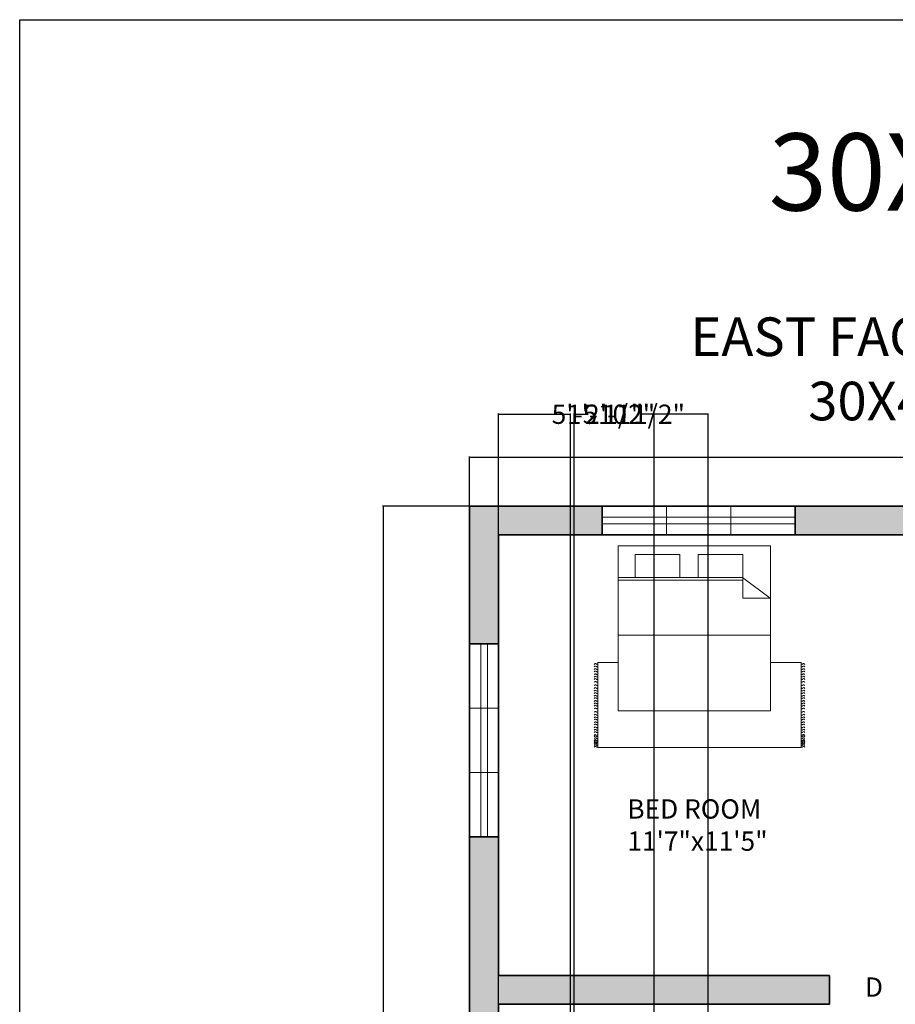
# Model space of a CAD drawing. Units: inches. Extents: x 2552 to 3196, y 4736 to 5443.
# Tile 5 of 8: x 2552 to 2824, y 5136 to 5443. Entities that reach past the tile are written whole.
import ezdxf

# ---------------------------------------------------------------- set-up
doc = ezdxf.new("R2010")
doc.units = ezdxf.units.IN
doc.header["$MEASUREMENT"] = 0
for name, color, linetype, lineweight in [('A-ANNO-DIMS', 2, 'Continuous', 18), ('A-ANNO-TTLB', 7, 'Continuous', 25), ('A-AREA-IDEN', 7, 'Continuous', 18), ('A-DOOR-IDEN', 7, 'Continuous', 18), ('A-FURN', 8, 'Continuous', 18), ('A-GLAZ', 4, 'Continuous', 18), ('A-WALL', 7, 'Continuous', 35)]:
    doc.layers.add(name, color=color, linetype=linetype, lineweight=lineweight)
doc.layers.add('A-WALL-PATT', color=30, linetype='Continuous', lineweight=13, true_color=0xf8991e)
doc.styles.get("Standard").update_dxf_attribs({"font": 'arial.ttf'})
doc.dimstyles.get("Standard").update_dxf_attribs({"dimtxt": 6, "dimasz": 0.18, "dimexe": 0.18, "dimexo": 0.0625, "dimgap": 0.09, "dimtad": 0, "dimtih": 1, "dimtoh": 1, "dimdec": 1, "dimzin": 0, "dimdsep": 46, "dimlunit": 3, "dimtxsty": 'Standard', "dimcen": 0.09, "dimadec": 0, "dimazin": 0, "dimtfac": 1, "dimtdec": 1, "dimtofl": 0, "dimtmove": 0, "dimatfit": 3, "dimfxl": 1, "dimtolj": 1, "dimtzin": 0, "dimarcsym": 0})

# ---------------------------------------------------------------- blocks, each defined once
blk = doc.blocks.new('*D1')
at = {"layer": 'A-ANNO-DIMS', "color": 0, "lineweight": -2, "transparency": 16777216}
for p, q in [((2691.59, 5291.32), (2664.57, 5291.32)), ((2664.75, 5291.14), (2664.75, 5052.97)), ((2664.75, 4808.5), (2664.75, 5046.66)), ((2691.59, 4808.32), (2664.57, 4808.32))]:
    blk.add_line(p, q, dxfattribs=at)
at = {"layer": 'A-ANNO-DIMS', "color": 0, "transparency": 16777216}
for points in [[(2664.72, 5291.14), (2664.78, 5291.14), (2664.75, 5291.32)], [(2664.72, 4808.5), (2664.78, 4808.5), (2664.75, 4808.32)]]:
    blk.add_solid(points, dxfattribs=at)
at = {"layer": 'Defpoints', "color": 0, "transparency": 16777216}
for p in [(2691.66, 5291.32), (2664.75, 4808.32), (2691.66, 4808.32)]:
    blk.add_point(p, dxfattribs=at)
at = {"layer": 'A-ANNO-DIMS', "color": 0, "transparency": 16777216, "insert": (2664.75, 5049.82), "char_height": 6, "attachment_point": 5}
blk.add_mtext('\\A1;40\'-3.0"', dxfattribs=at)
blk = doc.blocks.new('*D2')
at = {"layer": 'A-ANNO-DIMS', "color": 0, "lineweight": -2, "transparency": 16777216}
for p, q in [((2691.66, 5291.38), (2691.66, 5306.69)), ((2691.84, 5306.51), (2859.27, 5306.51)), ((3054.48, 5306.51), (2887.04, 5306.51)), ((3054.66, 5291.38), (3054.66, 5306.69))]:
    blk.add_line(p, q, dxfattribs=at)
at = {"layer": 'A-ANNO-DIMS', "color": 0, "transparency": 16777216}
for points in [[(2691.84, 5306.54), (2691.84, 5306.48), (2691.66, 5306.51)], [(3054.48, 5306.54), (3054.48, 5306.48), (3054.66, 5306.51)]]:
    blk.add_solid(points, dxfattribs=at)
at = {"layer": 'Defpoints', "color": 0, "transparency": 16777216}
for p in [(3054.66, 5306.51), (2691.66, 5291.32), (3054.66, 5291.32)]:
    blk.add_point(p, dxfattribs=at)
at = {"layer": 'A-ANNO-DIMS', "color": 0, "transparency": 16777216, "insert": (2873.16, 5306.51), "char_height": 6, "attachment_point": 5}
blk.add_mtext('\\A1;30\'-3.0"', dxfattribs=at)
blk = doc.blocks.new('WIN-60IN-THREE-LIGHT')
for p, q in [((60, 9), (0, 9)), ((20, 9), (20, 0)), ((40, 0), (40, 9)), ((60, 5.5), (0, 5.5)), ((0, 3.5), (60, 3.5)), ((0, 0), (60, 0))]:
    blk.add_line(p, q)
blk = doc.blocks.new('BED-DOUBLE')
for p, q in [((46.16, 52.82), (7.4, 52.82)), ((46.16, 52.82), (54.77, 46.47)), ((46.22, 52.82), (46.22, 46.47)), ((46.22, 52), (7.4, 52)), ((46.22, 46.47), (54.77, 46.47)), ((54.83, 34.96), (7.4, 34.96)), ((1.13, 0), (1.13, 26.37)), ((1.13, 26.37), (7.43, 26.37)), ((54.83, 26.37), (64.37, 26.37)), ((64.37, 26.37), (64.37, 0)), ((64.37, 0), (1.13, 0))]:
    blk.add_line(p, q)
for points in [[(54.83, 62.68), (54.83, 11.36), (7.4, 11.36), (7.4, 62.68)], [(26.65, 59.98), (26.65, 52.82), (12.75, 52.82), (12.75, 59.98)], [(46.22, 59.98), (46.22, 52.82), (32.32, 52.82), (32.32, 59.98)]]:
    blk.add_lwpolyline(points, close=True)
for points, knots in [([(0, 25.83), (0.1, 25.96), (0.29, 26.2), (0.63, 25.96), (0.91, 25.78), (1.06, 25.89), (1.13, 25.94)], [0, 0, 0, 0, 0.400747, 0.791423, 1.067667, 1.29709, 1.29709, 1.29709, 1.29709]), ([(0, 25.06), (0.1, 25.18), (0.29, 25.42), (0.63, 25.18), (0.91, 25), (1.06, 25.11), (1.13, 25.16)], [0, 0, 0, 0, 0.400747, 0.791423, 1.067667, 1.29709, 1.29709, 1.29709, 1.29709]), ([(0, 24.24), (0.1, 24.36), (0.29, 24.6), (0.63, 24.36), (0.91, 24.19), (1.06, 24.29), (1.13, 24.34)], [0, 0, 0, 0, 0.400747, 0.791423, 1.067667, 1.29709, 1.29709, 1.29709, 1.29709]), ([(65.48, 25.83), (65.39, 25.96), (65.19, 26.2), (64.85, 25.96), (64.57, 25.78), (64.42, 25.89), (64.36, 25.94)], [0, 0, 0, 0, 0.400747, 0.791423, 1.067667, 1.29709, 1.29709, 1.29709, 1.29709]), ([(65.48, 25.06), (65.39, 25.18), (65.19, 25.42), (64.85, 25.18), (64.57, 25), (64.42, 25.11), (64.36, 25.16)], [0, 0, 0, 0, 0.400747, 0.791423, 1.067667, 1.29709, 1.29709, 1.29709, 1.29709]), ([(65.48, 24.24), (65.39, 24.36), (65.19, 24.6), (64.85, 24.36), (64.57, 24.19), (64.42, 24.29), (64.36, 24.34)], [0, 0, 0, 0, 0.400747, 0.791423, 1.067667, 1.29709, 1.29709, 1.29709, 1.29709]), ([(0, 23.51), (0.1, 23.63), (0.29, 23.87), (0.63, 23.63), (0.91, 23.46), (1.06, 23.57), (1.13, 23.62)], [0, 0, 0, 0, 0.400747, 0.791423, 1.067667, 1.29709, 1.29709, 1.29709, 1.29709]), ([(0, 22.63), (0.1, 22.75), (0.29, 22.99), (0.63, 22.75), (0.91, 22.58), (1.06, 22.68), (1.13, 22.73)], [0, 0, 0, 0, 0.400747, 0.791423, 1.067667, 1.29709, 1.29709, 1.29709, 1.29709]), ([(0, 21.88), (0.1, 22), (0.29, 22.24), (0.63, 22), (0.91, 21.83), (1.06, 21.93), (1.13, 21.98)], [0, 0, 0, 0, 0.400747, 0.791423, 1.067667, 1.29709, 1.29709, 1.29709, 1.29709]), ([(65.48, 23.51), (65.39, 23.63), (65.19, 23.87), (64.85, 23.63), (64.57, 23.46), (64.42, 23.57), (64.36, 23.62)], [0, 0, 0, 0, 0.400747, 0.791423, 1.067667, 1.29709, 1.29709, 1.29709, 1.29709]), ([(65.48, 22.63), (65.39, 22.75), (65.19, 22.99), (64.85, 22.75), (64.57, 22.58), (64.42, 22.68), (64.36, 22.73)], [0, 0, 0, 0, 0.400747, 0.791423, 1.067667, 1.29709, 1.29709, 1.29709, 1.29709]), ([(65.48, 21.88), (65.39, 22), (65.19, 22.24), (64.85, 22), (64.57, 21.83), (64.42, 21.93), (64.36, 21.98)], [0, 0, 0, 0, 0.400747, 0.791423, 1.067667, 1.29709, 1.29709, 1.29709, 1.29709]), ([(0, 21.15), (0.1, 21.27), (0.29, 21.51), (0.63, 21.27), (0.91, 21.1), (1.06, 21.2), (1.13, 21.25)], [0, 0, 0, 0, 0.400747, 0.791423, 1.067667, 1.29709, 1.29709, 1.29709, 1.29709]), ([(0, 20.27), (0.1, 20.39), (0.29, 20.63), (0.63, 20.39), (0.91, 20.22), (1.06, 20.32), (1.13, 20.37)], [0, 0, 0, 0, 0.400747, 0.791423, 1.067667, 1.29709, 1.29709, 1.29709, 1.29709]), ([(0, 19.23), (0.1, 19.35), (0.29, 19.59), (0.63, 19.35), (0.91, 19.18), (1.06, 19.29), (1.13, 19.33)], [0, 0, 0, 0, 0.400747, 0.791423, 1.067667, 1.29709, 1.29709, 1.29709, 1.29709]), ([(0, 18.35), (0.1, 18.47), (0.29, 18.71), (0.63, 18.47), (0.91, 18.3), (1.06, 18.4), (1.13, 18.45)], [0, 0, 0, 0, 0.400747, 0.791423, 1.067667, 1.29709, 1.29709, 1.29709, 1.29709]), ([(65.48, 21.15), (65.39, 21.27), (65.19, 21.51), (64.85, 21.27), (64.57, 21.1), (64.42, 21.2), (64.36, 21.25)], [0, 0, 0, 0, 0.400747, 0.791423, 1.067667, 1.29709, 1.29709, 1.29709, 1.29709]), ([(65.48, 20.27), (65.39, 20.39), (65.19, 20.63), (64.85, 20.39), (64.57, 20.22), (64.42, 20.32), (64.36, 20.37)], [0, 0, 0, 0, 0.400747, 0.791423, 1.067667, 1.29709, 1.29709, 1.29709, 1.29709]), ([(65.48, 19.23), (65.39, 19.35), (65.19, 19.59), (64.85, 19.35), (64.57, 19.18), (64.42, 19.29), (64.36, 19.33)], [0, 0, 0, 0, 0.400747, 0.791423, 1.067667, 1.29709, 1.29709, 1.29709, 1.29709]), ([(65.48, 18.35), (65.39, 18.47), (65.19, 18.71), (64.85, 18.47), (64.57, 18.3), (64.42, 18.4), (64.36, 18.45)], [0, 0, 0, 0, 0.400747, 0.791423, 1.067667, 1.29709, 1.29709, 1.29709, 1.29709]), ([(0, 17.53), (0.1, 17.65), (0.29, 17.89), (0.63, 17.65), (0.91, 17.48), (1.06, 17.59), (1.13, 17.64)], [0, 0, 0, 0, 0.400747, 0.791423, 1.067667, 1.29709, 1.29709, 1.29709, 1.29709]), ([(0, 16.76), (0.1, 16.88), (0.29, 17.12), (0.63, 16.88), (0.91, 16.7), (1.06, 16.81), (1.13, 16.86)], [0, 0, 0, 0, 0.400747, 0.791423, 1.067667, 1.29709, 1.29709, 1.29709, 1.29709]), ([(0, 15.94), (0.1, 16.06), (0.29, 16.3), (0.63, 16.06), (0.91, 15.89), (1.06, 15.99), (1.13, 16.04)], [0, 0, 0, 0, 0.400747, 0.791423, 1.067667, 1.29709, 1.29709, 1.29709, 1.29709]), ([(0, 15.21), (0.1, 15.33), (0.29, 15.57), (0.63, 15.33), (0.91, 15.16), (1.06, 15.27), (1.13, 15.31)], [0, 0, 0, 0, 0.400747, 0.791423, 1.067667, 1.29709, 1.29709, 1.29709, 1.29709]), ([(65.48, 17.53), (65.39, 17.65), (65.19, 17.89), (64.85, 17.65), (64.57, 17.48), (64.42, 17.59), (64.36, 17.64)], [0, 0, 0, 0, 0.400747, 0.791423, 1.067667, 1.29709, 1.29709, 1.29709, 1.29709]), ([(65.48, 16.76), (65.39, 16.88), (65.19, 17.12), (64.85, 16.88), (64.57, 16.7), (64.42, 16.81), (64.36, 16.86)], [0, 0, 0, 0, 0.400747, 0.791423, 1.067667, 1.29709, 1.29709, 1.29709, 1.29709]), ([(65.48, 15.94), (65.39, 16.06), (65.19, 16.3), (64.85, 16.06), (64.57, 15.89), (64.42, 15.99), (64.36, 16.04)], [0, 0, 0, 0, 0.400747, 0.791423, 1.067667, 1.29709, 1.29709, 1.29709, 1.29709]), ([(65.48, 15.21), (65.39, 15.33), (65.19, 15.57), (64.85, 15.33), (64.57, 15.16), (64.42, 15.27), (64.36, 15.31)], [0, 0, 0, 0, 0.400747, 0.791423, 1.067667, 1.29709, 1.29709, 1.29709, 1.29709]), ([(0, 14.33), (0.1, 14.45), (0.29, 14.69), (0.63, 14.45), (0.91, 14.28), (1.06, 14.38), (1.13, 14.43)], [0, 0, 0, 0, 0.400747, 0.791423, 1.067667, 1.29709, 1.29709, 1.29709, 1.29709]), ([(0, 13.58), (0.1, 13.7), (0.29, 13.94), (0.63, 13.7), (0.91, 13.53), (1.06, 13.63), (1.13, 13.68)], [0, 0, 0, 0, 0.400747, 0.791423, 1.067667, 1.29709, 1.29709, 1.29709, 1.29709]), ([(0, 12.85), (0.1, 12.97), (0.29, 13.21), (0.63, 12.97), (0.91, 12.8), (1.06, 12.9), (1.13, 12.95)], [0, 0, 0, 0, 0.400747, 0.791423, 1.067667, 1.29709, 1.29709, 1.29709, 1.29709]), ([(65.48, 14.33), (65.39, 14.45), (65.19, 14.69), (64.85, 14.45), (64.57, 14.28), (64.42, 14.38), (64.36, 14.43)], [0, 0, 0, 0, 0.400747, 0.791423, 1.067667, 1.29709, 1.29709, 1.29709, 1.29709]), ([(65.48, 13.58), (65.39, 13.7), (65.19, 13.94), (64.85, 13.7), (64.57, 13.53), (64.42, 13.63), (64.36, 13.68)], [0, 0, 0, 0, 0.400747, 0.791423, 1.067667, 1.29709, 1.29709, 1.29709, 1.29709]), ([(65.48, 12.85), (65.39, 12.97), (65.19, 13.21), (64.85, 12.97), (64.57, 12.8), (64.42, 12.9), (64.36, 12.95)], [0, 0, 0, 0, 0.400747, 0.791423, 1.067667, 1.29709, 1.29709, 1.29709, 1.29709]), ([(0, 11.97), (0.1, 12.09), (0.29, 12.33), (0.63, 12.09), (0.91, 11.92), (1.06, 12.02), (1.13, 12.07)], [0, 0, 0, 0, 0.400747, 0.791423, 1.067667, 1.29709, 1.29709, 1.29709, 1.29709]), ([(0, 10.93), (0.1, 11.05), (0.29, 11.29), (0.63, 11.05), (0.91, 10.88), (1.06, 10.99), (1.13, 11.03)], [0, 0, 0, 0, 0.400747, 0.791423, 1.067667, 1.29709, 1.29709, 1.29709, 1.29709]), ([(0, 10.05), (0.1, 10.17), (0.29, 10.41), (0.63, 10.17), (0.91, 10), (1.06, 10.1), (1.13, 10.15)], [0, 0, 0, 0, 0.400747, 0.791423, 1.067667, 1.29709, 1.29709, 1.29709, 1.29709]), ([(0, 9.23), (0.1, 9.35), (0.29, 9.59), (0.63, 9.35), (0.91, 9.18), (1.06, 9.29), (1.13, 9.33)], [0, 0, 0, 0, 0.400747, 0.791423, 1.067667, 1.29709, 1.29709, 1.29709, 1.29709]), ([(65.48, 11.97), (65.39, 12.09), (65.19, 12.33), (64.85, 12.09), (64.57, 11.92), (64.42, 12.02), (64.36, 12.07)], [0, 0, 0, 0, 0.400747, 0.791423, 1.067667, 1.29709, 1.29709, 1.29709, 1.29709]), ([(65.48, 10.93), (65.39, 11.05), (65.19, 11.29), (64.85, 11.05), (64.57, 10.88), (64.42, 10.99), (64.36, 11.03)], [0, 0, 0, 0, 0.400747, 0.791423, 1.067667, 1.29709, 1.29709, 1.29709, 1.29709]), ([(65.48, 10.05), (65.39, 10.17), (65.19, 10.41), (64.85, 10.17), (64.57, 10), (64.42, 10.1), (64.36, 10.15)], [0, 0, 0, 0, 0.400747, 0.791423, 1.067667, 1.29709, 1.29709, 1.29709, 1.29709]), ([(65.48, 9.23), (65.39, 9.35), (65.19, 9.59), (64.85, 9.35), (64.57, 9.18), (64.42, 9.29), (64.36, 9.33)], [0, 0, 0, 0, 0.400747, 0.791423, 1.067667, 1.29709, 1.29709, 1.29709, 1.29709]), ([(0, 8.54), (0.1, 8.66), (0.29, 8.9), (0.63, 8.66), (0.91, 8.49), (1.06, 8.6), (1.13, 8.65)], [0, 0, 0, 0, 0.400747, 0.791423, 1.067667, 1.29709, 1.29709, 1.29709, 1.29709]), ([(0, 7.73), (0.1, 7.85), (0.29, 8.09), (0.63, 7.85), (0.91, 7.67), (1.06, 7.78), (1.13, 7.83)], [0, 0, 0, 0, 0.400747, 0.791423, 1.067667, 1.29709, 1.29709, 1.29709, 1.29709]), ([(0, 7), (0.1, 7.12), (0.29, 7.36), (0.63, 7.12), (0.91, 6.95), (1.06, 7.05), (1.13, 7.1)], [0, 0, 0, 0, 0.400747, 0.791423, 1.067667, 1.29709, 1.29709, 1.29709, 1.29709]), ([(0, 6.12), (0.1, 6.24), (0.29, 6.48), (0.63, 6.24), (0.91, 6.06), (1.06, 6.17), (1.13, 6.22)], [0, 0, 0, 0, 0.400747, 0.791423, 1.067667, 1.29709, 1.29709, 1.29709, 1.29709]), ([(65.48, 8.54), (65.39, 8.66), (65.19, 8.9), (64.85, 8.66), (64.57, 8.49), (64.42, 8.6), (64.36, 8.65)], [0, 0, 0, 0, 0.400747, 0.791423, 1.067667, 1.29709, 1.29709, 1.29709, 1.29709]), ([(65.48, 7.73), (65.39, 7.85), (65.19, 8.09), (64.85, 7.85), (64.57, 7.67), (64.42, 7.78), (64.36, 7.83)], [0, 0, 0, 0, 0.400747, 0.791423, 1.067667, 1.29709, 1.29709, 1.29709, 1.29709]), ([(65.48, 7), (65.39, 7.12), (65.19, 7.36), (64.85, 7.12), (64.57, 6.95), (64.42, 7.05), (64.36, 7.1)], [0, 0, 0, 0, 0.400747, 0.791423, 1.067667, 1.29709, 1.29709, 1.29709, 1.29709]), ([(65.48, 6.12), (65.39, 6.24), (65.19, 6.48), (64.85, 6.24), (64.57, 6.06), (64.42, 6.17), (64.36, 6.22)], [0, 0, 0, 0, 0.400747, 0.791423, 1.067667, 1.29709, 1.29709, 1.29709, 1.29709]), ([(0, 5.36), (0.1, 5.49), (0.29, 5.72), (0.63, 5.49), (0.91, 5.31), (1.06, 5.42), (1.13, 5.47)], [0, 0, 0, 0, 0.400747, 0.791423, 1.067667, 1.29709, 1.29709, 1.29709, 1.29709]), ([(0, 4.64), (0.1, 4.76), (0.29, 5), (0.63, 4.76), (0.91, 4.58), (1.06, 4.69), (1.13, 4.74)], [0, 0, 0, 0, 0.400747, 0.791423, 1.067667, 1.29709, 1.29709, 1.29709, 1.29709]), ([(0, 3.75), (0.1, 3.87), (0.29, 4.11), (0.63, 3.87), (0.91, 3.7), (1.06, 3.81), (1.13, 3.86)], [0, 0, 0, 0, 0.400747, 0.791423, 1.067667, 1.29709, 1.29709, 1.29709, 1.29709]), ([(0, 3.32), (0.1, 3.45), (0.29, 3.7), (0.63, 3.44), (0.91, 3.27), (1.06, 3.38), (1.13, 3.43)], [0, 0, 0, 0, 0.407265, 0.802015, 1.07826, 1.307683, 1.307683, 1.307683, 1.307683]), ([(65.48, 5.36), (65.39, 5.49), (65.19, 5.72), (64.85, 5.49), (64.57, 5.31), (64.42, 5.42), (64.36, 5.47)], [0, 0, 0, 0, 0.400747, 0.791423, 1.067667, 1.29709, 1.29709, 1.29709, 1.29709]), ([(65.48, 4.64), (65.39, 4.76), (65.19, 5), (64.85, 4.76), (64.58, 4.59), (64.43, 4.69), (64.37, 4.73)], [0, 0, 0, 0, 0.400747, 0.791423, 1.067667, 1.283686, 1.283686, 1.283686, 1.283686]), ([(65.48, 3.75), (65.39, 3.87), (65.19, 4.11), (64.85, 3.88), (64.58, 3.7), (64.43, 3.8), (64.37, 3.85)], [0, 0, 0, 0, 0.400747, 0.791423, 1.067667, 1.283686, 1.283686, 1.283686, 1.283686]), ([(65.48, 3.32), (65.39, 3.45), (65.19, 3.69), (64.85, 3.45), (64.58, 3.27), (64.43, 3.37), (64.37, 3.42)], [0, 0, 0, 0, 0.402903, 0.794912, 1.071156, 1.287177, 1.287177, 1.287177, 1.287177]), ([(0, 2.76), (0.1, 2.88), (0.29, 3.12), (0.63, 2.88), (0.91, 2.71), (1.06, 2.81), (1.13, 2.86)], [0, 0, 0, 0, 0.400747, 0.791423, 1.067667, 1.29709, 1.29709, 1.29709, 1.29709]), ([(0, 2.18), (0.1, 2.31), (0.29, 2.54), (0.63, 2.31), (0.91, 2.13), (1.06, 2.24), (1.13, 2.29)], [0, 0, 0, 0, 0.400747, 0.791423, 1.067667, 1.29709, 1.29709, 1.29709, 1.29709]), ([(0, 1.88), (0.1, 2), (0.29, 2.24), (0.63, 2), (0.91, 1.82), (1.06, 1.93), (1.13, 1.98)], [0, 0, 0, 0, 0.400747, 0.791423, 1.067667, 1.29709, 1.29709, 1.29709, 1.29709]), ([(0, 1.46), (0.1, 1.58), (0.29, 1.82), (0.63, 1.58), (0.91, 1.4), (1.06, 1.51), (1.13, 1.56)], [0, 0, 0, 0, 0.400747, 0.791423, 1.067667, 1.29709, 1.29709, 1.29709, 1.29709]), ([(0, 1.06), (0.1, 1.18), (0.29, 1.42), (0.63, 1.18), (0.91, 1.01), (1.06, 1.11), (1.13, 1.16)], [0, 0, 0, 0, 0.400747, 0.791423, 1.067667, 1.29709, 1.29709, 1.29709, 1.29709]), ([(0, 0.57), (0.1, 0.7), (0.29, 0.93), (0.63, 0.7), (0.91, 0.52), (1.06, 0.63), (1.13, 0.68)], [0, 0, 0, 0, 0.400747, 0.791423, 1.067667, 1.29709, 1.29709, 1.29709, 1.29709]), ([(0, 0.07), (0.1, 0.19), (0.29, 0.43), (0.63, 0.19), (0.91, 0.02), (1.06, 0.13), (1.13, 0.17)], [0, 0, 0, 0, 0.400747, 0.791423, 1.067667, 1.29709, 1.29709, 1.29709, 1.29709]), ([(65.48, 1.43), (65.39, 1.55), (65.19, 1.79), (64.85, 1.55), (64.57, 1.38), (64.42, 1.48), (64.36, 1.53)], [0, 0, 0, 0, 0.400747, 0.791423, 1.067667, 1.29709, 1.29709, 1.29709, 1.29709]), ([(65.48, 1.03), (65.39, 1.15), (65.19, 1.39), (64.85, 1.15), (64.57, 0.98), (64.42, 1.09), (64.36, 1.13)], [0, 0, 0, 0, 0.400747, 0.791423, 1.067667, 1.29709, 1.29709, 1.29709, 1.29709]), ([(65.48, 0.55), (65.39, 0.67), (65.19, 0.91), (64.85, 0.67), (64.57, 0.49), (64.42, 0.6), (64.36, 0.65)], [0, 0, 0, 0, 0.400747, 0.791423, 1.067667, 1.29709, 1.29709, 1.29709, 1.29709]), ([(65.48, 0.07), (65.39, 0.19), (65.19, 0.43), (64.85, 0.19), (64.57, 0.02), (64.42, 0.13), (64.36, 0.17)], [0, 0, 0, 0, 0.400747, 0.791423, 1.067667, 1.29709, 1.29709, 1.29709, 1.29709]), ([(65.48, 2.73), (65.39, 2.85), (65.19, 3.09), (64.85, 2.85), (64.58, 2.68), (64.43, 2.78), (64.37, 2.82)], [0, 0, 0, 0, 0.400747, 0.791423, 1.067667, 1.283686, 1.283686, 1.283686, 1.283686]), ([(65.48, 2.16), (65.39, 2.28), (65.19, 2.52), (64.85, 2.28), (64.58, 2.11), (64.43, 2.21), (64.37, 2.25)], [0, 0, 0, 0, 0.400747, 0.791423, 1.067667, 1.283686, 1.283686, 1.283686, 1.283686]), ([(65.48, 1.85), (65.39, 1.97), (65.19, 2.21), (64.85, 1.97), (64.58, 1.8), (64.43, 1.9), (64.37, 1.94)], [0, 0, 0, 0, 0.400747, 0.791423, 1.067667, 1.283686, 1.283686, 1.283686, 1.283686])]:
    blk.add_open_spline(points, degree=3, knots=knots)
blk = doc.blocks.new('*D29')
at = {"layer": 'A-ANNO-DIMS', "color": 0, "lineweight": -2, "transparency": 16777216}
for p, q in [((2724.14, 5033.79), (2724.14, 5320.05)), ((2724.32, 5319.87), (2728.51, 5319.87)), ((2748.94, 5319.87), (2744.75, 5319.87)), ((2749.12, 5033.79), (2749.12, 5320.05))]:
    blk.add_line(p, q, dxfattribs=at)
at = {"layer": 'A-ANNO-DIMS', "color": 0, "transparency": 16777216}
for points in [[(2724.32, 5319.9), (2724.32, 5319.84), (2724.14, 5319.87)], [(2748.94, 5319.9), (2748.94, 5319.84), (2749.12, 5319.87)]]:
    blk.add_solid(points, dxfattribs=at)
at = {"layer": 'Defpoints', "color": 0, "transparency": 16777216}
for p in [(2749.12, 5319.87), (2724.14, 5033.73), (2749.12, 5033.73)]:
    blk.add_point(p, dxfattribs=at)
at = {"layer": 'A-ANNO-DIMS', "color": 0, "transparency": 16777216, "insert": (2736.63, 5319.87), "char_height": 6, "attachment_point": 5}
blk.add_mtext('\\A1;2\'-1"', dxfattribs=at)
blk = doc.blocks.new('*D37')
at = {"layer": 'A-ANNO-DIMS', "color": 0, "lineweight": -2, "transparency": 16777216}
for p, q in [((2700.66, 4902.38), (2700.66, 5320.05)), ((2700.84, 5319.87), (2722.83, 5319.87)), ((2723.01, 4902.38), (2723.01, 5320.05)), ((2723.01, 5319.87), (2723.19, 5319.87))]:
    blk.add_line(p, q, dxfattribs=at)
at = {"layer": 'A-ANNO-DIMS', "color": 0, "transparency": 16777216}
for points in [[(2700.84, 5319.9), (2700.84, 5319.84), (2700.66, 5319.87)], [(2722.83, 5319.9), (2722.83, 5319.84), (2723.01, 5319.87)]]:
    blk.add_solid(points, dxfattribs=at)
at = {"layer": 'Defpoints', "color": 0, "transparency": 16777216}
for p in [(2723.01, 5319.87), (2700.66, 4902.32), (2723.01, 4902.32)]:
    blk.add_point(p, dxfattribs=at)
at = {"layer": 'A-ANNO-DIMS', "color": 0, "transparency": 16777216, "insert": (2740.29, 5319.87), "char_height": 6, "attachment_point": 5}
blk.add_mtext('\\A1;1\'-10 1/2"', dxfattribs=at)
blk = doc.blocks.new('*D40')
at = {"layer": 'A-ANNO-DIMS', "color": 0, "lineweight": -2, "transparency": 16777216}
for p, q in [((2700.66, 4947.38), (2700.66, 5320.05)), ((2700.84, 5319.87), (2718.23, 5319.87)), ((2765.73, 5319.87), (2748.34, 5319.87)), ((2765.91, 4947.38), (2765.91, 5320.05))]:
    blk.add_line(p, q, dxfattribs=at)
at = {"layer": 'A-ANNO-DIMS', "color": 0, "transparency": 16777216}
for points in [[(2700.84, 5319.9), (2700.84, 5319.84), (2700.66, 5319.87)], [(2765.73, 5319.9), (2765.73, 5319.84), (2765.91, 5319.87)]]:
    blk.add_solid(points, dxfattribs=at)
at = {"layer": 'Defpoints', "color": 0, "transparency": 16777216}
for p in [(2765.91, 5319.87), (2700.66, 4947.32), (2765.91, 4947.32)]:
    blk.add_point(p, dxfattribs=at)
at = {"layer": 'A-ANNO-DIMS', "color": 0, "transparency": 16777216, "insert": (2733.28, 5319.87), "char_height": 6, "attachment_point": 5}
blk.add_mtext('\\A1;5\'-5 1/2"', dxfattribs=at)

msp = doc.modelspace()

# ---------------------------------------------------------------- hatches: boundary and pattern name
at = {"layer": 'A-WALL-PATT'}
h = msp.add_hatch(color=256, dxfattribs=at)
h.dxf.hatch_style = 1
h.paths.add_polyline_path([(2700.66, 5282.32), (2732.91, 5282.32), (2732.91, 5291.32), (2691.66, 5291.32), (2691.66, 5248.4), (2700.66, 5248.4)])
h.paths.add_polyline_path([(2865.22, 5291.32), (2792.91, 5291.32), (2792.91, 5282.32), (2839.66, 5282.32), (2839.66, 5136.32), (2848.66, 5136.32), (2848.66, 5182.32), (2913.66, 5182.32), (2913.66, 5246.32), (2904.66, 5246.32), (2904.66, 5191.32), (2848.66, 5191.32), (2848.66, 5282.32), (2865.22, 5282.32)])
h.paths.add_polyline_path([(2946.08, 5291.32), (2889.22, 5291.32), (2889.22, 5282.32), (2946.08, 5282.32)])
h.paths.add_polyline_path([(3054.66, 5291.32), (3006.08, 5291.32), (3006.08, 5282.32), (3045.66, 5282.32), (3045.66, 5249.18), (3054.66, 5249.18)])
h.paths.add_polyline_path([(3054.66, 5189.18), (3045.66, 5189.18), (3045.66, 5145.32), (2904.66, 5145.32), (2904.66, 5136.32), (3045.66, 5136.32), (3045.66, 5103.54), (3054.66, 5103.54)])
h.paths.add_polyline_path([(3054.66, 5043.54), (3045.66, 5043.54), (3045.66, 5012.32), (2913.66, 5012.32), (2913.66, 5100.32), (2904.66, 5100.32), (2904.66, 5003.32), (3045.66, 5003.32), (3045.66, 4980.34), (3054.66, 4980.34)])
h.paths.add_polyline_path([(3054.66, 4920.34), (3045.66, 4920.34), (3045.66, 4886.32), (3029.6, 4886.32), (3029.6, 4877.32), (3045.66, 4877.32), (3045.66, 4817.32), (3041.59, 4817.32), (3041.59, 4808.32), (3054.66, 4808.32)])
h.paths.add_polyline_path([(2996.66, 4877.32), (3013.11, 4877.32), (3013.11, 4886.32), (2987.66, 4886.32), (2987.66, 4808.32), (2999.73, 4808.32), (2999.73, 4817.32), (2996.66, 4817.32)])
h.paths.add_polyline_path([(2825.66, 4877.32), (2853.9, 4877.32), (2853.9, 4886.32), (2825.66, 4886.32), (2825.66, 5000.12), (2816.66, 5000.12), (2816.66, 4817.32), (2785.76, 4817.32), (2785.76, 4808.32), (2825.66, 4808.32)])
h.paths.add_polyline_path([(2951.66, 4886.32), (2913.9, 4886.32), (2913.9, 4877.32), (2951.66, 4877.32)])
h.paths.add_polyline_path([(2725.76, 4817.32), (2700.66, 4817.32), (2700.66, 4833.17), (2691.66, 4833.17), (2691.66, 4808.32), (2725.76, 4808.32)])
h.paths.add_polyline_path([(2700.66, 4902.32), (2691.66, 4902.32), (2691.66, 4869.17), (2700.66, 4869.17)])
h.paths.add_polyline_path([(2765.91, 4947.32), (2700.66, 4947.32), (2700.66, 4977.71), (2691.66, 4977.71), (2691.66, 4938.32), (2765.91, 4938.32)])
h.paths.add_polyline_path([(2825.66, 5077.32), (2773.66, 5077.32), (2773.66, 5112.32), (2764.66, 5112.32), (2764.66, 5077.32), (2700.66, 5077.32), (2700.66, 5102.51), (2691.66, 5102.51), (2691.66, 5037.71), (2700.66, 5037.71), (2700.66, 5068.32), (2816.66, 5068.32), (2816.66, 5036.12), (2825.66, 5036.12)])
h.paths.add_polyline_path([(2803.66, 5145.32), (2700.66, 5145.32), (2700.66, 5188.4), (2691.66, 5188.4), (2691.66, 5126.51), (2700.66, 5126.51), (2700.66, 5136.32), (2803.66, 5136.32)])

# ---------------------------------------------------------------- linework, layer by layer
at = {"layer": 'A-ANNO-TTLB'}
msp.add_lwpolyline([(2551.65, 5442.6), (3195.75, 5442.6), (3195.75, 4736.32), (2551.65, 4736.32)], close=True, dxfattribs=at)
at = {"layer": 'A-WALL'}
for p, q in [((2691.66, 5291.32), (3054.66, 5291.32)), ((2691.66, 5291.32), (2691.66, 4938.32)), ((2732.91, 5291.32), (2732.91, 5282.32)), ((2792.91, 5282.32), (2792.91, 5291.32)), ((2700.66, 5282.32), (2700.66, 5145.32)), ((2700.66, 5282.32), (2839.66, 5282.32)), ((2691.66, 5248.4), (2700.66, 5248.4)), ((2700.66, 5188.4), (2691.66, 5188.4)), ((2700.66, 5145.32), (2803.66, 5145.32)), ((2803.66, 5136.32), (2803.66, 5145.32)), ((2700.66, 5136.32), (2803.66, 5136.32)), ((2700.66, 5136.32), (2700.66, 5077.32))]:
    msp.add_line(p, q, dxfattribs=at)

# ---------------------------------------------------------------- block references
at = {"layer": 'A-FURN'}
msp.add_blockref('BED-DOUBLE', (2730.44, 5216.23), dxfattribs=at)
at = {"layer": 'A-GLAZ'}
msp.add_blockref('WIN-60IN-THREE-LIGHT', (2732.91, 5282.32), dxfattribs=at)
at = {"layer": 'A-GLAZ', "rotation": 89.99999999999818}
msp.add_blockref('WIN-60IN-THREE-LIGHT', (2700.66, 5188.4), dxfattribs=at)

# ---------------------------------------------------------------- texts
at = {"layer": 'A-ANNO-TTLB', "attachment_point": 1}
for s, width, insert, char_height in [('30X40 FEET', 248.7494, (2784.71, 5407.23), 24), ('EAST FACING HOUSE PLAN\\P          30X40 FEET', 240.3543, (2760.34, 5349.98), 12)]:
    msp.add_mtext_dynamic_manual_height_columns(s, width=width, gutter_width=1, heights=[0], dxfattribs=dict(at, insert=insert, char_height=char_height))
at = {"layer": 'A-AREA-IDEN', "insert": (2740.72, 5200.08), "char_height": 6, "attachment_point": 1}
msp.add_mtext_dynamic_manual_height_columns('BED ROOM \\P11\'7"x11\'5"', width=104.0705, gutter_width=1, heights=[0], dxfattribs=at)
at = {"layer": 'A-DOOR-IDEN', "insert": (2814.63, 5144.67), "char_height": 6, "attachment_point": 1}
msp.add_mtext_dynamic_manual_height_columns('D', width=10.2167, gutter_width=1, heights=[0], dxfattribs=at)

# ---------------------------------------------------------------- dimensions: what is measured, and where the dimension line sits
at = {"layer": 'A-ANNO-DIMS'}
for base, p1, p2, override, picture, middle in [((2723.00559, 5319.86809), (2700.65555, 4902.31809), (2723.00559, 4902.31809), {"dimdec": 1, "dimlfac": 1, "dimrnd": 0, "dimzin": 1, "dimdsep": 46, "dimlunit": 4, "dimfrac": 2}, '*D37', (2740.28923, 5319.86809)), ((2765.9115, 5319.8681), (2700.6556, 4947.3181), (2765.9115, 4947.3181), {"dimdec": 1, "dimlfac": 1, "dimrnd": 0, "dimzin": 1, "dimdsep": 46, "dimlunit": 4, "dimfrac": 2}, '*D40', (2733.2835, 5319.8681)), ((2749.12, 5319.87), (2724.14, 5033.73), (2749.12, 5033.73), {"dimdec": 1, "dimlfac": 1, "dimrnd": 0, "dimzin": 1, "dimdsep": 46, "dimlunit": 4, "dimfrac": 2}, '*D29', (2736.63, 5319.87)), ((3054.66, 5306.51), (2691.66, 5291.32), (3054.66, 5291.32), {"dimclrd": 0, "dimclre": 0, "dimclrt": 0}, '*D2', (2873.16, 5306.51))]:
    dim = msp.add_linear_dim(base=base, p1=p1, p2=p2, dimstyle='Standard', override=override, dxfattribs=at)
    dim.commit()
    dim.dimension.update_dxf_attribs({"geometry": picture, "text_midpoint": middle})
dim = msp.add_linear_dim(base=(2664.75, 4808.32), p1=(2691.66, 5291.32), p2=(2691.66, 4808.32), angle=90, dimstyle='Standard', override={"dimclrd": 0, "dimclre": 0, "dimclrt": 0}, dxfattribs=at)
dim.commit()
dim.dimension.update_dxf_attribs({"geometry": '*D1', "text_midpoint": (2664.75, 5049.82)})

doc.saveas('drawing.dxf')
